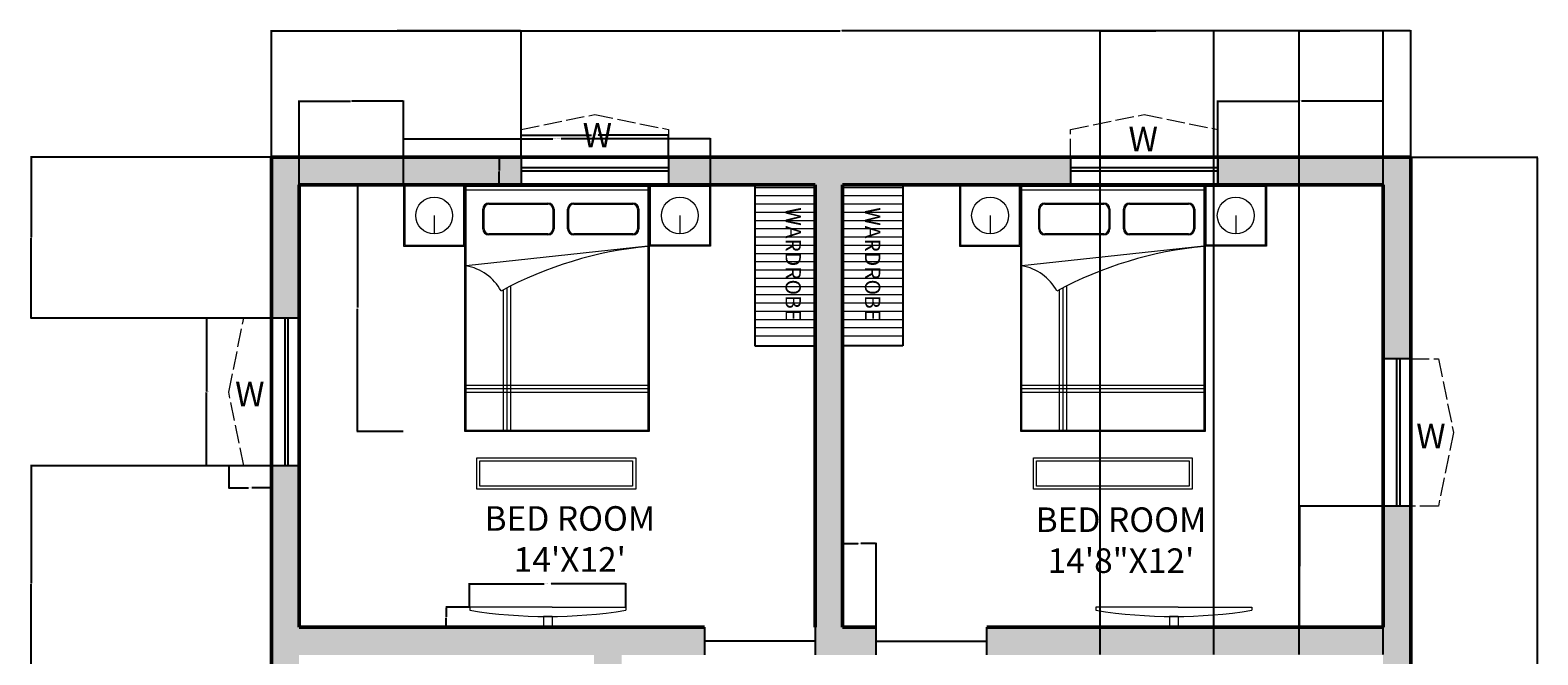
# Model space of a CAD drawing. Units: inches. Extents: x -75 to 416, y -487 to 70.
# Tile 5 of 5: x -75 to 416, y -133 to 70. Entities that reach past the tile are written whole.
import ezdxf

# ---------------------------------------------------------------- set-up
doc = ezdxf.new("R2010")
doc.units = ezdxf.units.IN
doc.header["$MEASUREMENT"] = 0
doc.linetypes.add('ACAD_ISO02W100', pattern=[15, 12, -3])
for name, color, linetype, lineweight in [('A-ANNO-DIMS', 2, 'Continuous', 18), ('A-ANNO-TEXT', 7, 'Continuous', 18), ('A-AREA-IDEN', 7, 'Continuous', 25), ('A-DOOR', 3, 'Continuous', 25), ('A-EQPM', 8, 'Continuous', 18), ('A-FLOR-CASE', 8, 'Continuous', 25), ('A-FLOR-CASE-PATT', 252, 'Continuous', 13), ('A-FURN', 8, 'Continuous', 18), ('A-GLAZ', 4, 'Continuous', 25), ('A-GLAZ-OVHD', 4, 'ACAD_ISO02W100', 13), ('A-WALL', 7, 'Continuous', 50), ('A-WALL-PATT', 252, 'Continuous', 13)]:
    doc.layers.add(name, color=color, linetype=linetype, lineweight=lineweight)
doc.styles.get("Standard").update_dxf_attribs({"font": 'arial.ttf'})
doc.dimstyles.get("Standard").update_dxf_attribs({"dimtxt": 0.18, "dimasz": 0.18, "dimexe": 0.18, "dimexo": 0.0625, "dimgap": 0.09, "dimtad": 0, "dimtih": 1, "dimtoh": 1, "dimdec": 4, "dimzin": 0, "dimdsep": 46, "dimtxsty": 'Standard', "dimcen": 0.09, "dimadec": 0, "dimazin": 0, "dimtfac": 1, "dimtdec": 4, "dimtofl": 0, "dimtmove": 0, "dimatfit": 3, "dimfxl": 1, "dimtolj": 1, "dimtzin": 0, "dimarcsym": 0})

# ---------------------------------------------------------------- blocks, each defined once
blk = doc.blocks.new('A$C0EA4476A')
at = {"linetype": 'ByBlock', "lineweight": -2}
for p, q in [((0, 2.008), (0, 1.508)), ((0.5, 2.008), (0, 2.008)), ((0.01, 1.998), (0.01, 1.518)), ((0.49, 1.998), (0.01, 1.998)), ((0.49, 1.518), (0.49, 1.998)), ((0.5, 2.008), (2, 2.008)), ((0.5, 0), (0.5, 2.008)), ((0.5, 1.508), (0.5, 2.008)), ((0.51, 1.998), (1.99, 1.998)), ((0.51, 0.01), (0.51, 1.998)), ((0.51, 1.968), (1.99, 1.968)), ((1.99, 1.998), (1.99, 0.01)), ((2, 2.008), (2, 0)), ((2, 2.008), (2.5, 2.008)), ((2, 1.508), (2, 2.008)), ((2.01, 1.998), (2.49, 1.998)), ((2.01, 1.518), (2.01, 1.998)), ((2.49, 1.998), (2.49, 1.518)), ((2.5, 2.008), (2.5, 1.508)), ((0.696, 1.86), (1.176, 1.86)), ((0.696, 1.85), (1.176, 1.85)), ((1.386, 1.86), (1.866, 1.86)), ((1.386, 1.85), (1.866, 1.85)), ((0.25, 1.758), (0.25, 1.608)), ((0.646, 1.65), (0.646, 1.81)), ((0.656, 1.65), (0.656, 1.81)), ((1.216, 1.81), (1.216, 1.65)), ((1.226, 1.81), (1.226, 1.65)), ((1.336, 1.65), (1.336, 1.81)), ((1.346, 1.65), (1.346, 1.81)), ((1.906, 1.81), (1.906, 1.65)), ((1.916, 1.81), (1.916, 1.65)), ((2.25, 1.758), (2.25, 1.608)), ((1.176, 1.61), (0.696, 1.61)), ((1.176, 1.6), (0.696, 1.6)), ((1.866, 1.61), (1.386, 1.61)), ((1.866, 1.6), (1.386, 1.6)), ((0, 1.508), (0.5, 1.508)), ((0.01, 1.518), (0.49, 1.518)), ((1.99, 1.508), (0.51, 1.349)), ((2.5, 1.508), (2, 1.508)), ((2.49, 1.518), (2.01, 1.518)), ((0.812, 1.153), (0.812, 0.01)), ((0.842, 1.169), (0.842, 0.01)), ((0.872, 1.184), (0.872, 0.01)), ((0.51, 0.377), (1.99, 0.377)), ((0.51, 0.35), (1.99, 0.35)), ((0.51, 0.322), (1.99, 0.322)), ((1.99, 0.01), (0.51, 0.01)), ((2, 0), (0.5, 0))]:
    blk.add_line(p, q, dxfattribs=at)
for centre in [(0.25, 1.758), (2.25, 1.758)]:
    blk.add_circle(centre, 0.15, dxfattribs=at)
for centre, radius, start, end in [((0.696, 1.81), 0.05, 90, 180), ((0.696, 1.81), 0.04, 90, 180), ((1.176, 1.81), 0.05, 0, 90), ((1.176, 1.81), 0.04, 0, 90), ((1.386, 1.81), 0.05, 90, 180), ((1.386, 1.81), 0.04, 90, 180), ((1.866, 1.81), 0.05, 0, 90), ((1.866, 1.81), 0.04, 0, 90), ((0.696, 1.65), 0.05, 180, 270), ((0.696, 1.65), 0.04, 180, 270), ((1.176, 1.65), 0.04, 270, 0), ((1.176, 1.65), 0.05, 270, 0), ((1.386, 1.65), 0.05, 180, 270), ((1.386, 1.65), 0.04, 180, 270), ((1.866, 1.65), 0.05, 270, 0), ((1.866, 1.65), 0.04, 270, 0), ((2.293, -1.636), 3.158, 95.5104, 118.3399), ((0.44, 0.952), 0.403, 28.4688, 79.9557)]:
    blk.add_arc(centre, radius, start, end, dxfattribs=at)
blk = doc.blocks.new('A$C1A706E3E')
blk.add_blockref('A$C0EA4476A', (0, 0))
blk = doc.blocks.new('WIN-48IN')
for p, q in [((0, 9), (0, 0)), ((48, 5.5), (0, 5.5)), ((48, 9), (48, 0)), ((48, 4.5), (0, 4.5))]:
    blk.add_line(p, q)
blk = doc.blocks.new('WIN-SHADE-48IN')
at = {"ltscale": 0.5}
for p, q in [((0, 4.91), (0, 13.91)), ((48, 13.91), (48, 4.91)), ((24, 0), (0, 4.91)), ((48, 4.91), (24, 0))]:
    blk.add_line(p, q, dxfattribs=at)
blk = doc.blocks.new('DOOR-36IN')
for p, q in [((0, 9), (0, 0)), ((36, 9), (36, 0)), ((36, 4.5), (0, 4.5))]:
    blk.add_line(p, q)
blk = doc.blocks.new('TV-WALL-MOUNT')
for p, q in [((24, 6.49), (0, 6.49)), ((0, 6.49), (0, 5.49)), ((26.81, 6.49), (24, 6.49)), ((26.81, 6.49), (50.81, 6.49)), ((50.81, 6.49), (50.81, 5.49)), ((24, 3.49), (24, 0)), ((26.81, 3.49), (24, 3.49)), ((26.81, 3.49), (26.81, 0))]:
    blk.add_line(p, q)
blk.add_arc((25.41, 165.85), 162.36, 260.9976, 279.0024)
blk = doc.blocks.new('BENCH-BED-END')
for points in [[(0, 10.24), (51.71, 10.24), (51.71, 0), (0, 0)], [(1, 9.24), (50.71, 9.24), (50.71, 1), (1, 1)]]:
    blk.add_lwpolyline(points, close=True)
blk = doc.blocks.new('WARDROBE-OUTLINE')
for p, q in [((0, 52.38), (0, 0)), ((0, 0), (19.56, 0))]:
    blk.add_line(p, q)
blk = doc.blocks.new('*D14')
at = {"layer": 'A-ANNO-DIMS', "color": 0, "lineweight": -2, "transparency": 16777216}
for p, q in [((84.86, 28.69), (84.86, 36.01)), ((85.04, 35.83), (107.74, 35.83)), ((132.68, 35.83), (109.98, 35.83)), ((132.86, 28.69), (132.86, 36.01))]:
    blk.add_line(p, q, dxfattribs=at)
at = {"layer": 'A-ANNO-DIMS', "color": 0, "transparency": 16777216}
for points in [[(85.04, 35.86), (85.04, 35.8), (84.86, 35.83)], [(132.68, 35.86), (132.68, 35.8), (132.86, 35.83)]]:
    blk.add_solid(points, dxfattribs=at)
at = {"layer": 'Defpoints', "color": 0, "transparency": 16777216}
for p in [(132.86, 35.83), (84.86, 28.63), (132.86, 28.63)]:
    blk.add_point(p, dxfattribs=at)
at = {"layer": 'A-ANNO-DIMS', "color": 0, "transparency": 16777216, "insert": (108.86, 35.83), "char_height": 0.18, "attachment_point": 5}
blk.add_mtext('\\A1;WINDOW 48 TYP.', dxfattribs=at)
blk = doc.blocks.new('*D15')
at = {"layer": 'A-ANNO-DIMS', "color": 0, "lineweight": -2, "transparency": 16777216}
for p, q in [((84.8, 28.63), (77.48, 28.63)), ((77.66, 28.45), (77.66, 24.31)), ((77.66, 19.81), (77.66, 23.94)), ((84.8, 19.63), (77.48, 19.63))]:
    blk.add_line(p, q, dxfattribs=at)
at = {"layer": 'A-ANNO-DIMS', "color": 0, "transparency": 16777216}
for points in [[(77.63, 28.45), (77.69, 28.45), (77.66, 28.63)], [(77.63, 19.81), (77.69, 19.81), (77.66, 19.63)]]:
    blk.add_solid(points, dxfattribs=at)
at = {"layer": 'Defpoints', "color": 0, "transparency": 16777216}
for p in [(77.66, 28.63), (84.86, 28.63), (84.86, 19.63)]:
    blk.add_point(p, dxfattribs=at)
at = {"layer": 'A-ANNO-DIMS', "color": 0, "transparency": 16777216, "insert": (77.66, 24.13), "char_height": 0.18, "attachment_point": 5}
blk.add_mtext('\\A1;9 TYP.', dxfattribs=at)
blk = doc.blocks.new('*D16')
at = {"layer": 'A-ANNO-DIMS', "color": 0, "lineweight": -2, "transparency": 16777216}
for p, q in [((-10.42, -23.81), (-17.74, -23.81)), ((-17.56, -23.99), (-17.56, -47.63)), ((-17.56, -71.63), (-17.56, -48)), ((-10.42, -71.81), (-17.74, -71.81))]:
    blk.add_line(p, q, dxfattribs=at)
at = {"layer": 'A-ANNO-DIMS', "color": 0, "transparency": 16777216}
for points in [[(-17.59, -23.99), (-17.53, -23.99), (-17.56, -23.81)], [(-17.59, -71.63), (-17.53, -71.63), (-17.56, -71.81)]]:
    blk.add_solid(points, dxfattribs=at)
at = {"layer": 'Defpoints', "color": 0, "transparency": 16777216}
for p in [(-10.36, -23.81), (-17.56, -71.81), (-10.36, -71.81)]:
    blk.add_point(p, dxfattribs=at)
at = {"layer": 'A-ANNO-DIMS', "color": 0, "transparency": 16777216, "insert": (-17.56, -47.81), "char_height": 0.18, "attachment_point": 5}
blk.add_mtext('\\A1;SHADE 48 TYP.', dxfattribs=at)
blk = doc.blocks.new('*D17')
at = {"layer": 'A-ANNO-DIMS', "color": 0, "lineweight": -2, "transparency": 16777216}
for p, q in [((-10.36, -71.88), (-10.36, -79.19)), ((3.55, -71.88), (3.55, -79.19)), ((-10.18, -79.01), (-3.92, -79.01)), ((3.37, -79.01), (-2.88, -79.01))]:
    blk.add_line(p, q, dxfattribs=at)
at = {"layer": 'A-ANNO-DIMS', "color": 0, "transparency": 16777216}
for points in [[(-10.18, -78.98), (-10.18, -79.04), (-10.36, -79.01)], [(3.37, -78.98), (3.37, -79.04), (3.55, -79.01)]]:
    blk.add_solid(points, dxfattribs=at)
at = {"layer": 'Defpoints', "color": 0, "transparency": 16777216}
for p in [(-10.36, -71.81), (3.55, -71.81), (3.55, -79.01)]:
    blk.add_point(p, dxfattribs=at)
at = {"layer": 'A-ANNO-DIMS', "color": 0, "transparency": 16777216, "insert": (-3.4, -79.01), "char_height": 0.18, "attachment_point": 5}
blk.add_mtext('\\A1;14 TYP.', dxfattribs=at)
blk = doc.blocks.new('*D20')
at = {"layer": 'A-ANNO-DIMS', "color": 0, "lineweight": -2, "transparency": 16777216}
for p, q in [((46.55, 19.69), (46.55, 34.81)), ((46.73, 34.63), (95.17, 34.63)), ((146.37, 34.63), (97.94, 34.63)), ((146.55, 19.69), (146.55, 34.81))]:
    blk.add_line(p, q, dxfattribs=at)
at = {"layer": 'A-ANNO-DIMS', "color": 0, "transparency": 16777216}
for points in [[(46.73, 34.66), (46.73, 34.6), (46.55, 34.63)], [(146.37, 34.66), (146.37, 34.6), (146.55, 34.63)]]:
    blk.add_solid(points, dxfattribs=at)
at = {"layer": 'Defpoints', "color": 0, "transparency": 16777216}
for p in [(146.55, 34.63), (46.55, 19.63), (146.55, 19.63)]:
    blk.add_point(p, dxfattribs=at)
at = {"layer": 'A-ANNO-DIMS', "color": 0, "transparency": 16777216, "insert": (96.55, 34.63), "char_height": 0.18, "attachment_point": 5}
blk.add_mtext('\\A1;BED GROUP 100 TYP.', dxfattribs=at)
blk = doc.blocks.new('*D21')
at = {"layer": 'A-ANNO-DIMS', "color": 0, "lineweight": -2, "transparency": 16777216}
for p, q in [((46.49, 19.63), (31.37, 19.63)), ((31.55, 19.45), (31.55, -20.35)), ((31.55, -60.51), (31.55, -20.72)), ((46.49, -60.69), (31.37, -60.69))]:
    blk.add_line(p, q, dxfattribs=at)
at = {"layer": 'A-ANNO-DIMS', "color": 0, "transparency": 16777216}
for points in [[(31.52, 19.45), (31.58, 19.45), (31.55, 19.63)], [(31.52, -60.51), (31.58, -60.51), (31.55, -60.69)]]:
    blk.add_solid(points, dxfattribs=at)
at = {"layer": 'Defpoints', "color": 0, "transparency": 16777216}
for p in [(31.55, 19.63), (46.55, 19.63), (46.55, -60.69)]:
    blk.add_point(p, dxfattribs=at)
at = {"layer": 'A-ANNO-DIMS', "color": 0, "transparency": 16777216, "insert": (31.55, -20.53), "char_height": 0.18, "attachment_point": 5}
blk.add_mtext('\\A1;80 TYP.', dxfattribs=at)
blk = doc.blocks.new('*D22')
at = {"layer": 'A-ANNO-DIMS', "color": 0, "lineweight": -2, "transparency": 16777216}
for p, q in [((68.1, -117.82), (68.1, -110.08)), ((68.28, -110.26), (92.41, -110.26)), ((118.74, -110.26), (94.62, -110.26)), ((118.92, -117.82), (118.92, -110.08))]:
    blk.add_line(p, q, dxfattribs=at)
at = {"layer": 'A-ANNO-DIMS', "color": 0, "transparency": 16777216}
for points in [[(68.28, -110.23), (68.28, -110.29), (68.1, -110.26)], [(118.74, -110.23), (118.74, -110.29), (118.92, -110.26)]]:
    blk.add_solid(points, dxfattribs=at)
at = {"layer": 'Defpoints', "color": 0, "transparency": 16777216}
for p in [(118.92, -110.26), (68.1, -117.88), (118.92, -117.88)]:
    blk.add_point(p, dxfattribs=at)
at = {"layer": 'A-ANNO-DIMS', "color": 0, "transparency": 16777216, "insert": (93.51, -110.26), "char_height": 0.18, "attachment_point": 5}
blk.add_mtext('\\A1;WALL TV 51 TYP.', dxfattribs=at)
blk = doc.blocks.new('*D23')
at = {"layer": 'A-ANNO-DIMS', "color": 0, "lineweight": -2, "transparency": 16777216}
for p, q in [((68.04, -117.88), (60.3, -117.88)), ((60.48, -118.06), (60.48, -120.95)), ((60.48, -124.19), (60.48, -121.31)), ((68.04, -124.37), (60.3, -124.37))]:
    blk.add_line(p, q, dxfattribs=at)
at = {"layer": 'A-ANNO-DIMS', "color": 0, "transparency": 16777216}
for points in [[(60.45, -118.06), (60.51, -118.06), (60.48, -117.88)], [(60.45, -124.19), (60.51, -124.19), (60.48, -124.37)]]:
    blk.add_solid(points, dxfattribs=at)
at = {"layer": 'Defpoints', "color": 0, "transparency": 16777216}
for p in [(60.48, -117.88), (68.1, -117.88), (68.1, -124.37)]:
    blk.add_point(p, dxfattribs=at)
at = {"layer": 'A-ANNO-DIMS', "color": 0, "transparency": 16777216, "insert": (60.48, -121.13), "char_height": 0.18, "attachment_point": 5}
blk.add_mtext('\\A1;6 TYP.', dxfattribs=at)
blk = doc.blocks.new('*D34')
at = {"layer": 'A-ANNO-DIMS', "color": 0, "lineweight": -2, "transparency": 16777216}
for p, q in [((3.55, 28.69), (3.55, 69.98)), ((3.73, 69.8), (188.78, 69.8)), ((374.37, 69.8), (189.32, 69.8)), ((374.55, 28.69), (374.55, 69.98))]:
    blk.add_line(p, q, dxfattribs=at)
at = {"layer": 'A-ANNO-DIMS', "color": 0, "transparency": 16777216}
for points in [[(3.73, 69.83), (3.73, 69.77), (3.55, 69.8)], [(374.37, 69.83), (374.37, 69.77), (374.55, 69.8)]]:
    blk.add_solid(points, dxfattribs=at)
at = {"layer": 'Defpoints', "color": 0, "transparency": 16777216}
for p in [(374.55, 69.8), (3.55, 28.63), (374.55, 28.63)]:
    blk.add_point(p, dxfattribs=at)
at = {"layer": 'A-ANNO-DIMS', "color": 0, "transparency": 16777216, "insert": (189.05, 69.8), "char_height": 0.18, "attachment_point": 5}
blk.add_mtext('\\A1;371', dxfattribs=at)
blk = doc.blocks.new('*D35')
at = {"layer": 'A-ANNO-DIMS', "color": 0, "lineweight": -2, "transparency": 16777216}
for p, q in [((374.615553, 28.625508), (415.902741, 28.625508)), ((415.722741, 28.445508), (415.722741, -208.194492)), ((415.722741, -445.194492), (415.722741, -208.554492)), ((374.615553, -445.374492), (415.902741, -445.374492))]:
    blk.add_line(p, q, dxfattribs=at)
at = {"layer": 'A-ANNO-DIMS', "color": 0, "transparency": 16777216}
for points in [[(415.692741, 28.445508), (415.752741, 28.445508), (415.722741, 28.625508)], [(415.692741, -445.194492), (415.752741, -445.194492), (415.722741, -445.374492)]]:
    blk.add_solid(points, dxfattribs=at)
at = {"layer": 'Defpoints', "color": 0, "transparency": 16777216}
for p in [(374.553053, 28.625508), (374.553053, -445.374492), (415.722741, -445.374492)]:
    blk.add_point(p, dxfattribs=at)
at = {"layer": 'A-ANNO-DIMS', "color": 0, "transparency": 16777216, "insert": (415.722741, -208.374492), "char_height": 0.18, "attachment_point": 5}
blk.add_mtext('\\A1;474', dxfattribs=at)
blk = doc.blocks.new('*D38')
at = {"layer": 'A-ANNO-DIMS', "color": 0, "lineweight": -2, "transparency": 16777216}
for p, q in [((3.55, 28.69), (3.55, 69.98)), ((3.73, 69.8), (43.88, 69.8)), ((84.68, 69.8), (44.53, 69.8)), ((84.86, 28.69), (84.86, 69.98))]:
    blk.add_line(p, q, dxfattribs=at)
at = {"layer": 'A-ANNO-DIMS', "color": 0, "transparency": 16777216}
for points in [[(3.73, 69.83), (3.73, 69.77), (3.55, 69.8)], [(84.68, 69.83), (84.68, 69.77), (84.86, 69.8)]]:
    blk.add_solid(points, dxfattribs=at)
at = {"layer": 'Defpoints', "color": 0, "transparency": 16777216}
for p in [(84.86, 69.8), (3.55, 28.63), (84.86, 28.63)]:
    blk.add_point(p, dxfattribs=at)
at = {"layer": 'A-ANNO-DIMS', "color": 0, "transparency": 16777216, "insert": (44.21, 69.8), "char_height": 0.18, "attachment_point": 5}
blk.add_mtext('\\A1;81.3', dxfattribs=at)
blk = doc.blocks.new('*D39')
at = {"layer": 'A-ANNO-DIMS', "color": 0, "lineweight": -2, "transparency": 16777216}
for p, q in [((311.74, 19.69), (311.74, 47.07)), ((311.92, 46.89), (338.27, 46.89)), ((365.37, 46.89), (339.02, 46.89)), ((365.55, 19.69), (365.55, 47.07))]:
    blk.add_line(p, q, dxfattribs=at)
at = {"layer": 'A-ANNO-DIMS', "color": 0, "transparency": 16777216}
for points in [[(311.92, 46.92), (311.92, 46.86), (311.74, 46.89)], [(365.37, 46.92), (365.37, 46.86), (365.55, 46.89)]]:
    blk.add_solid(points, dxfattribs=at)
at = {"layer": 'Defpoints', "color": 0, "transparency": 16777216}
for p in [(365.55, 46.89), (311.74, 19.63), (365.55, 19.63)]:
    blk.add_point(p, dxfattribs=at)
at = {"layer": 'A-ANNO-DIMS', "color": 0, "transparency": 16777216, "insert": (338.65, 46.89), "char_height": 0.18, "attachment_point": 5}
blk.add_mtext('\\A1;53.81', dxfattribs=at)
blk = doc.blocks.new('*D40')
at = {"layer": 'A-ANNO-DIMS', "color": 0, "lineweight": -2, "transparency": 16777216}
for p, q in [((365.49, -85.02), (338.11, -85.02)), ((338.29, -85.2), (338.29, -104.51)), ((338.29, -124.19), (338.29, -104.88)), ((365.49, -124.37), (338.11, -124.37))]:
    blk.add_line(p, q, dxfattribs=at)
at = {"layer": 'A-ANNO-DIMS', "color": 0, "transparency": 16777216}
for points in [[(338.26, -85.2), (338.32, -85.2), (338.29, -85.02)], [(338.26, -124.19), (338.32, -124.19), (338.29, -124.37)]]:
    blk.add_solid(points, dxfattribs=at)
at = {"layer": 'Defpoints', "color": 0, "transparency": 16777216}
for p in [(338.29, -85.02), (365.55, -85.02), (365.55, -124.37)]:
    blk.add_point(p, dxfattribs=at)
at = {"layer": 'A-ANNO-DIMS', "color": 0, "transparency": 16777216, "insert": (338.29, -104.7), "char_height": 0.18, "attachment_point": 5}
blk.add_mtext('\\A1;39.355', dxfattribs=at)
blk = doc.blocks.new('*D43')
at = {"layer": 'A-ANNO-DIMS', "color": 0, "lineweight": -2, "transparency": 16777216}
for p, q in [((3.49, 28.63), (-74.89, 28.63)), ((-74.71, 28.45), (-74.71, 2.59)), ((-74.71, -23.63), (-74.71, 2.22)), ((3.49, -23.81), (-74.89, -23.81))]:
    blk.add_line(p, q, dxfattribs=at)
at = {"layer": 'A-ANNO-DIMS', "color": 0, "transparency": 16777216}
for points in [[(-74.74, 28.45), (-74.68, 28.45), (-74.71, 28.63)], [(-74.74, -23.63), (-74.68, -23.63), (-74.71, -23.81)]]:
    blk.add_solid(points, dxfattribs=at)
at = {"layer": 'Defpoints', "color": 0, "transparency": 16777216}
for p in [(3.55, 28.63), (-74.71, -23.81), (3.55, -23.81)]:
    blk.add_point(p, dxfattribs=at)
at = {"layer": 'A-ANNO-DIMS', "color": 0, "transparency": 16777216, "insert": (-74.71, 2.41), "char_height": 0.18, "attachment_point": 5}
blk.add_mtext('\\A1;52.44', dxfattribs=at)
blk = doc.blocks.new('*D44')
at = {"layer": 'A-ANNO-DIMS', "color": 0, "lineweight": -2, "transparency": 16777216}
for p, q in [((3.49, -71.81), (-74.89, -71.81)), ((-74.71, -71.99), (-74.71, -110.05)), ((-74.71, -148.46), (-74.71, -110.41)), ((3.49, -148.64), (-74.89, -148.64))]:
    blk.add_line(p, q, dxfattribs=at)
at = {"layer": 'A-ANNO-DIMS', "color": 0, "transparency": 16777216}
for points in [[(-74.74, -71.99), (-74.68, -71.99), (-74.71, -71.81)], [(-74.74, -148.46), (-74.68, -148.46), (-74.71, -148.64)]]:
    blk.add_solid(points, dxfattribs=at)
at = {"layer": 'Defpoints', "color": 0, "transparency": 16777216}
for p in [(3.55, -71.81), (-74.71, -148.64), (3.55, -148.64)]:
    blk.add_point(p, dxfattribs=at)
at = {"layer": 'A-ANNO-DIMS', "color": 0, "transparency": 16777216, "insert": (-74.71, -110.23), "char_height": 0.18, "attachment_point": 5}
blk.add_mtext('\\A1;76.83', dxfattribs=at)
blk = doc.blocks.new('*D54')
at = {"layer": 'A-ANNO-DIMS', "color": 0, "lineweight": -2, "transparency": 16777216}
for p, q in [((338.22, -133.31), (338.22, 69.98)), ((338.4, 69.8), (351.49, 69.8)), ((365.37, 69.8), (352.28, 69.8)), ((365.55, -133.31), (365.55, 69.98))]:
    blk.add_line(p, q, dxfattribs=at)
at = {"layer": 'A-ANNO-DIMS', "color": 0, "transparency": 16777216}
for points in [[(338.4, 69.83), (338.4, 69.77), (338.22, 69.8)], [(365.37, 69.83), (365.37, 69.77), (365.55, 69.8)]]:
    blk.add_solid(points, dxfattribs=at)
at = {"layer": 'Defpoints', "color": 0, "transparency": 16777216}
for p in [(365.55, 69.8), (338.22, -133.37), (365.55, -133.37)]:
    blk.add_point(p, dxfattribs=at)
at = {"layer": 'A-ANNO-DIMS', "color": 0, "transparency": 16777216, "insert": (351.89, 69.8), "char_height": 0.18, "attachment_point": 5}
blk.add_mtext('\\A1;27.33', dxfattribs=at)
blk = doc.blocks.new('*D57')
at = {"layer": 'A-ANNO-DIMS', "color": 0, "lineweight": -2, "transparency": 16777216}
for p, q in [((189.55, -124.31), (189.55, -96.93)), ((189.73, -97.11), (194.56, -97.11)), ((200.29, -97.11), (195.46, -97.11)), ((200.47, -124.31), (200.47, -96.93))]:
    blk.add_line(p, q, dxfattribs=at)
at = {"layer": 'A-ANNO-DIMS', "color": 0, "transparency": 16777216}
for points in [[(189.73, -97.08), (189.73, -97.14), (189.55, -97.11)], [(200.29, -97.08), (200.29, -97.14), (200.47, -97.11)]]:
    blk.add_solid(points, dxfattribs=at)
at = {"layer": 'Defpoints', "color": 0, "transparency": 16777216}
for p in [(200.47, -97.11), (189.55, -124.37), (200.47, -124.37)]:
    blk.add_point(p, dxfattribs=at)
at = {"layer": 'A-ANNO-DIMS', "color": 0, "transparency": 16777216, "insert": (195.01, -97.11), "char_height": 0.18, "attachment_point": 5}
blk.add_mtext('\\A1;10.914', dxfattribs=at)
blk = doc.blocks.new('*D59')
at = {"layer": 'A-ANNO-DIMS', "color": 0, "lineweight": -2, "transparency": 16777216}
for p, q in [((12.55, 19.69), (12.55, 47.07)), ((12.73, 46.89), (29.33, 46.89)), ((46.37, 46.89), (29.77, 46.89)), ((46.55, 19.69), (46.55, 47.07))]:
    blk.add_line(p, q, dxfattribs=at)
at = {"layer": 'A-ANNO-DIMS', "color": 0, "transparency": 16777216}
for points in [[(12.73, 46.92), (12.73, 46.86), (12.55, 46.89)], [(46.37, 46.92), (46.37, 46.86), (46.55, 46.89)]]:
    blk.add_solid(points, dxfattribs=at)
at = {"layer": 'Defpoints', "color": 0, "transparency": 16777216}
for p in [(46.55, 46.89), (12.55, 19.63), (46.55, 19.63)]:
    blk.add_point(p, dxfattribs=at)
at = {"layer": 'A-ANNO-DIMS', "color": 0, "transparency": 16777216, "insert": (29.55, 46.89), "char_height": 0.18, "attachment_point": 5}
blk.add_mtext('\\A1;34', dxfattribs=at)
blk = doc.blocks.new('*D66')
at = {"layer": 'A-ANNO-DIMS', "color": 0, "lineweight": -2, "transparency": 16777216}
for p, q in [((273.46, -133.31), (273.46, 69.98)), ((273.64, 69.8), (291.5, 69.8)), ((310.28, 69.8), (292.43, 69.8)), ((310.46, -133.31), (310.46, 69.98))]:
    blk.add_line(p, q, dxfattribs=at)
at = {"layer": 'A-ANNO-DIMS', "color": 0, "transparency": 16777216}
for points in [[(273.64, 69.83), (273.64, 69.77), (273.46, 69.8)], [(310.28, 69.83), (310.28, 69.77), (310.46, 69.8)]]:
    blk.add_solid(points, dxfattribs=at)
at = {"layer": 'Defpoints', "color": 0, "transparency": 16777216}
for p in [(310.46, 69.8), (273.46, -133.37), (310.46, -133.37)]:
    blk.add_point(p, dxfattribs=at)
at = {"layer": 'A-ANNO-DIMS', "color": 0, "transparency": 16777216, "insert": (291.96, 69.8), "char_height": 0.18, "attachment_point": 5}
blk.add_mtext('\\A1;37.004', dxfattribs=at)

msp = doc.modelspace()

# ---------------------------------------------------------------- hatches: boundary and pattern name
at = {"layer": 'A-FLOR-CASE-PATT'}
h = msp.add_hatch(dxfattribs=at)
h.set_pattern_fill('ANSI31', color=256, scale=21.476, angle=-45, style=0)
h.paths.add_polyline_path([(160.9968, -31.4078), (180.5531, -31.4078), (180.5531, 19.5977), (160.9968, 19.5977)])
h = msp.add_hatch(dxfattribs=at)
h.set_pattern_fill('ANSI31', color=256, scale=21.476, angle=-45, style=0)
h.paths.add_polyline_path([(189.5531, -31.4078), (209.1093, -31.4078), (209.1093, 19.5977), (189.5531, 19.5977)])
at = {"layer": 'A-WALL-PATT'}
h = msp.add_hatch(color=256, dxfattribs=at)
h.dxf.hatch_style = 1
h.paths.add_polyline_path([(84.8603, 28.6255), (3.5531, 28.6255), (3.5531, -23.8141), (12.5531, -23.8141), (12.5531, 19.6255), (84.8603, 19.6255)])
h.paths.add_polyline_path([(263.7442, 28.6255), (132.8603, 28.6255), (132.8603, 19.6255), (146.5531, 19.6255), (180.5531, 19.6255), (180.5531, -124.3745), (180.5531, -133.3745), (200.467, -133.3745), (200.467, -124.3745), (189.5531, -124.3745), (189.5531, 19.6255), (263.7442, 19.6255)])
h.paths.add_polyline_path([(374.5531, 28.6255), (311.7442, 28.6255), (311.7442, 19.6255), (327.5531, 19.6255), (365.5531, 19.6255), (365.5531, -37.0191), (374.5531, -37.0191)])
h.paths.add_polyline_path([(144.5531, -124.3745), (12.5531, -124.3745), (12.5531, -71.8141), (3.5531, -71.8141), (3.5531, -148.6403), (12.5531, -148.6403), (12.5531, -133.3745), (144.5531, -133.3745)])
h.paths.add_polyline_path([(117.5531, -133.3745), (108.5531, -133.3745), (108.5531, -161.7866), (117.5531, -161.7866)])
h.paths.add_polyline_path([(374.5531, -85.0191), (365.5531, -85.0191), (365.5531, -124.3745), (236.467, -124.3745), (236.467, -133.3745), (374.5531, -133.3745)])
h.paths.add_polyline_path([(374.5531, -133.3745), (365.5531, -133.3745), (365.5531, -183.1692), (374.5531, -183.1692)])
h.paths.add_polyline_path([(374.5531, -231.1692), (365.5531, -231.1692), (365.5531, -265.3745), (260.5531, -265.3745), (260.5531, -274.3745), (374.5531, -274.3745)])
h.paths.add_polyline_path([(260.5531, -265.3745), (215.5531, -265.3745), (215.5531, -288.4908), (224.5531, -288.4908), (224.5531, -274.3745), (260.5531, -274.3745)])
h.paths.add_polyline_path([(374.5531, -274.3745), (365.5531, -274.3745), (365.5531, -345.9302), (374.5531, -345.9302)])
h.paths.add_polyline_path([(374.5531, -393.9302), (365.5531, -393.9302), (365.5531, -436.3745), (321.1982, -436.3745), (321.1982, -445.3745), (374.5531, -445.3745)])
h.paths.add_polyline_path([(224.5531, -324.4908), (215.5531, -324.4908), (215.5531, -445.3745), (273.1982, -445.3745), (273.1982, -436.3745), (265.0531, -436.3745), (245.0531, -436.3745), (224.5531, -436.3745)])
h.paths.add_polyline_path([(12.5531, -183.233), (3.5531, -183.233), (3.5531, -214.3745), (117.5531, -214.3745), (117.5531, -197.7866), (108.5531, -197.7866), (108.5531, -205.3745), (12.5531, -205.3745)])
h.paths.add_polyline_path([(12.5531, -214.3745), (3.5531, -214.3745), (3.5531, -290.2477), (12.5531, -290.2477)])
h.paths.add_polyline_path([(75.0426, -381.3745), (12.5531, -381.3745), (12.5531, -350.2477), (3.5531, -350.2477), (3.5531, -390.3745), (75.0426, -390.3745)])
h.paths.add_polyline_path([(154.4537, -381.3745), (123.0426, -381.3745), (123.0426, -390.3745), (154.4537, -390.3745)])
h.paths.add_polyline_path([(215.5531, -381.3745), (202.4537, -381.3745), (202.4537, -390.3745), (215.5531, -390.3745)])

# ---------------------------------------------------------------- linework, layer by layer
at = {"layer": 'A-WALL'}
for p, q in [((3.5531, 28.6255), (374.5531, 28.6255)), ((3.5531, 28.6255), (3.5531, -390.3745)), ((374.5531, 28.6255), (374.5531, -445.3745)), ((12.5531, 19.6255), (180.5531, 19.6255)), ((12.5531, 19.6255), (12.5531, -124.3745)), ((180.5531, 19.6255), (180.5531, -124.3745)), ((189.5531, 19.6255), (189.5531, -124.3745)), ((189.5531, 19.6255), (365.5531, 19.6255)), ((365.5531, 19.6255), (365.5531, -124.3745)), ((12.5531, -124.3745), (144.5531, -124.3745)), ((189.5531, -124.3745), (200.467, -124.3745)), ((236.467, -124.3745), (365.5531, -124.3745))]:
    msp.add_line(p, q, dxfattribs=at)

# ---------------------------------------------------------------- block references
at = {"layer": 'A-DOOR'}
msp.add_blockref('DOOR-36IN', (144.553, -133.374), dxfattribs=at)
at = {"layer": 'A-DOOR', "rotation": 180}
msp.add_blockref('DOOR-36IN', (236.467, -124.375), dxfattribs=at)
at = {"layer": 'A-EQPM'}
for p in [(68.1051, -124.374), (272.017, -124.374)]:
    msp.add_blockref('TV-WALL-MOUNT', p, dxfattribs=at)
at = {"layer": 'A-FLOR-CASE'}
msp.add_blockref('WARDROBE-OUTLINE', (160.997, -32.75), dxfattribs=at)
at = {"layer": 'A-FLOR-CASE', "extrusion": (0, 0, -1), "zscale": -1}
msp.add_blockref('WARDROBE-OUTLINE', (-209.1091, -32.75), dxfattribs=at)
at = {"layer": 'A-FURN', "xscale": 40.00000000000001, "yscale": 40.00000000000001, "zscale": 40.00000000000001}
for p in [(46.5531, -60.6945), (227.5531, -60.6945)]:
    msp.add_blockref('A$C1A706E3E', p, dxfattribs=at)
at = {"layer": 'A-FURN'}
for p in [(70.462, -79.489), (251.6997, -79.489)]:
    msp.add_blockref('BENCH-BED-END', p, dxfattribs=at)
at = {"layer": 'A-GLAZ'}
for p in [(84.8607, 19.626), (263.7447, 19.626)]:
    msp.add_blockref('WIN-48IN', p, dxfattribs=at)
at = {"layer": 'A-GLAZ', "rotation": 270.0000000000002}
for p in [(3.5535, -23.8146), (365.5535, -37.0196)]:
    msp.add_blockref('WIN-48IN', p, dxfattribs=at)
at = {"layer": 'A-GLAZ-OVHD'}
for p, rotation in [((132.8605, 42.535), 180), ((311.7444, 42.535), 180), ((-10.3565, -23.8139), 270), ((388.4626, -85.0194), 89.99999999999984)]:
    msp.add_blockref('WIN-SHADE-48IN', p, dxfattribs=dict(at, rotation=rotation))

# ---------------------------------------------------------------- texts
at = {"layer": 'A-ANNO-TEXT', "char_height": 8, "attachment_point": 1}
for insert in [(102.1175, 39.7855), (279.859, 38.5215), (-11.055, -44.4745), (373.5427, -58.1108)]:
    msp.add_mtext_dynamic_manual_height_columns('\\pxqc;W', width=15.130285, gutter_width=1, heights=[0], dxfattribs=dict(at, insert=insert))
at = {"layer": 'A-ANNO-TEXT', "char_height": 5, "attachment_point": 1, "rotation": 270}
for insert in [(175.9489, 65.9505), (201.8138, 65.9505)]:
    msp.add_mtext_dynamic_manual_height_columns('\\pxqc;WARDROBE', width=144.357858, gutter_width=1, heights=[0], dxfattribs=dict(at, insert=insert))
at = {"layer": 'A-AREA-IDEN', "char_height": 8, "attachment_point": 1}
for s, insert in [("\\pxqc;BED ROOM\\P14'X12'", (28.5411, -84.9859)), ('\\pxqc;BED ROOM\\P14\'8"X12\'', (207.9997, -85.3813))]:
    msp.add_mtext_dynamic_manual_height_columns(s, width=144.357858, gutter_width=1, heights=[0], dxfattribs=dict(at, insert=insert))

# ---------------------------------------------------------------- dimensions: what is measured, and where the dimension line sits
at = {"layer": 'A-ANNO-DIMS'}
for base, p1, p2, override, picture, middle in [((374.5531, 69.7952), (3.5531, 28.6255), (374.5531, 28.6255), {"dimdec": 0, "dimlfac": 1, "dimrnd": 0, "dimzin": 0, "dimdsep": 46, "dimlunit": 2}, '*D34', (189.0531, 69.7952)), ((84.8603, 69.7952), (3.5531, 28.6255), (84.8603, 28.6255), {"dimdec": 1, "dimlfac": 1, "dimrnd": 0, "dimzin": 0, "dimdsep": 46, "dimlunit": 2}, '*D38', (44.2067, 69.7952)), ((310.465, 69.7952), (273.461, -133.3745), (310.465, -133.3745), {"dimdec": 3, "dimlfac": 1, "dimrnd": 0, "dimzin": 0, "dimdsep": 46, "dimlunit": 2}, '*D66', (291.963, 69.7952)), ((365.5531, 69.7952), (338.2223, -133.3745), (365.5531, -133.3745), {"dimdec": 2, "dimlfac": 1, "dimrnd": 0, "dimzin": 0, "dimdsep": 46, "dimlunit": 2}, '*D54', (351.8877, 69.7952))]:
    dim = msp.add_linear_dim(base=base, p1=p1, p2=p2, dimstyle='Standard', override=override, dxfattribs=at)
    dim.commit()
    dim.dimension.update_dxf_attribs({"geometry": picture, "text_midpoint": middle})
for base, p1, p2, angle, override, picture, middle in [((46.5531, 46.8855), (12.5531, 19.6255), (46.5531, 19.6255), 0, {"dimdec": 0, "dimlfac": 1, "dimrnd": 0, "dimzin": 0, "dimdsep": 46, "dimlunit": 2}, '*D59', (29.5531, 46.8855)), ((365.5531, 46.8855), (311.7442, 19.6255), (365.5531, 19.6255), 0, {"dimdec": 2, "dimlfac": 1, "dimrnd": 0, "dimzin": 0, "dimdsep": 46, "dimlunit": 2}, '*D39', (338.6486, 46.8855)), ((-74.7069, -23.8141), (3.5531, 28.6255), (3.5531, -23.8141), 90, {"dimdec": 2, "dimlfac": 1, "dimrnd": 0, "dimzin": 0, "dimdsep": 46, "dimlunit": 2}, '*D43', (-74.7069, 2.4057)), ((415.7227, -445.3745), (374.5531, 28.6255), (374.5531, -445.3745), 90, {"dimdec": 0, "dimlfac": 1, "dimrnd": 0, "dimzin": 0, "dimdsep": 46, "dimlunit": 2}, '*D35', (415.7227, -208.3745)), ((-74.7069, -148.6403), (3.5531, -71.8141), (3.5531, -148.6403), 90, {"dimdec": 2, "dimlfac": 1, "dimrnd": 0, "dimzin": 0, "dimdsep": 46, "dimlunit": 2}, '*D44', (-74.7069, -110.2272)), ((338.2931, -85.0191), (365.5531, -124.3745), (365.5531, -85.0191), 90, {"dimdec": 3, "dimlfac": 1, "dimrnd": 0, "dimzin": 0, "dimdsep": 46, "dimlunit": 2}, '*D40', (338.2931, -104.6968)), ((200.467, -97.1145), (189.5531, -124.3745), (200.467, -124.3745), 0, {"dimdec": 3, "dimlfac": 1, "dimrnd": 0, "dimzin": 0, "dimdsep": 46, "dimlunit": 2}, '*D57', (195.01, -97.1145))]:
    dim = msp.add_linear_dim(base=base, p1=p1, p2=p2, angle=angle, dimstyle='Standard', override=override, dxfattribs=at)
    dim.commit()
    dim.dimension.update_dxf_attribs({"geometry": picture, "text_midpoint": middle})
for base, p1, p2, text, picture, middle in [((146.5531, 34.6255), (46.5531, 19.6255), (146.5531, 19.6255), 'BED GROUP <> TYP.', '*D20', (96.5531, 34.6255)), ((132.8603, 35.8255), (84.8603, 28.6255), (132.8603, 28.6255), 'WINDOW <> TYP.', '*D14', (108.8603, 35.8255)), ((3.5531, -79.0141), (-10.3566, -71.8141), (3.5531, -71.8141), '<> TYP.', '*D17', (-3.4018, -79.0141)), ((118.916, -110.2612), (68.105, -117.8829), (118.916, -117.8829), 'WALL TV <> TYP.', '*D22', (93.5105, -110.2612))]:
    dim = msp.add_linear_dim(base=base, p1=p1, p2=p2, text=text, dimstyle='Standard', override={"dimdec": 0, "dimlfac": 1, "dimrnd": 0, "dimzin": 0, "dimdsep": 46, "dimlunit": 2}, dxfattribs=at)
    dim.commit()
    dim.dimension.update_dxf_attribs({"geometry": picture, "text_midpoint": middle})
for base, p1, p2, angle, text, picture, middle in [((77.6603, 28.6255), (84.8603, 19.6255), (84.8603, 28.6255), 90, '<> TYP.', '*D15', (77.6603, 24.1255)), ((31.5531, 19.6255), (46.5531, -60.6945), (46.5531, 19.6255), 90, '<> TYP.', '*D21', (31.5531, -20.5345)), ((-17.5566, -71.8141), (-10.3566, -23.8141), (-10.3566, -71.8141), 270, 'SHADE <> TYP.', '*D16', (-17.5566, -47.8141)), ((60.4833, -117.8829), (68.105, -124.3745), (68.105, -117.8829), 90, '<> TYP.', '*D23', (60.4833, -121.1287))]:
    dim = msp.add_linear_dim(base=base, p1=p1, p2=p2, angle=angle, text=text, dimstyle='Standard', override={"dimdec": 0, "dimlfac": 1, "dimrnd": 0, "dimzin": 0, "dimdsep": 46, "dimlunit": 2}, dxfattribs=at)
    dim.commit()
    dim.dimension.update_dxf_attribs({"geometry": picture, "text_midpoint": middle})

doc.saveas('drawing.dxf')
